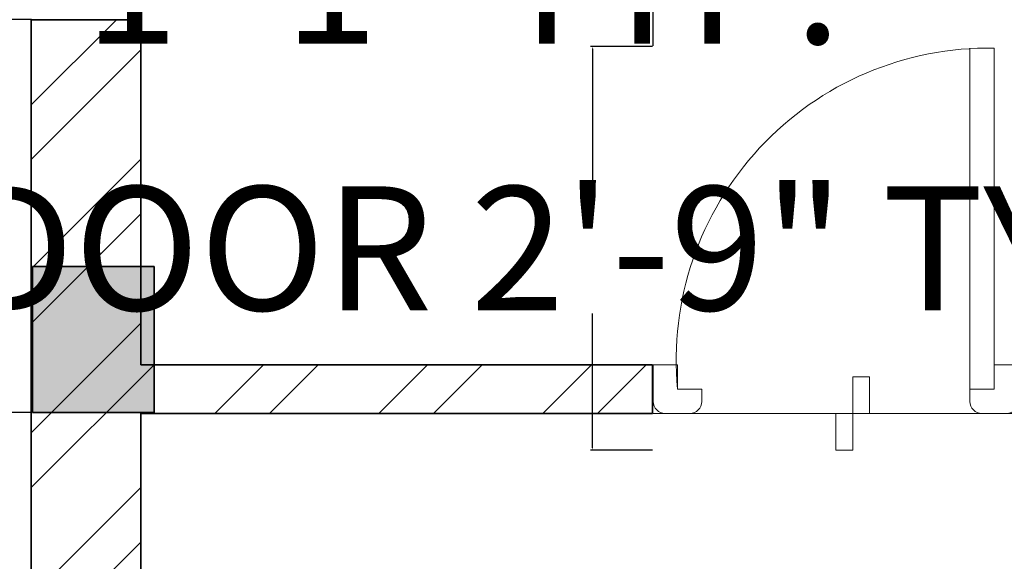
# Model space of a CAD drawing. Units: inches. Extents: x 1812 to 2791, y 2306 to 2959.
# Tile 6 of 8: x 2453 to 2534, y 2748 to 2793. Entities that reach past the tile are written whole.
import ezdxf

# ---------------------------------------------------------------- set-up
doc = ezdxf.new("R2010")
doc.units = ezdxf.units.IN
doc.layers.get('Defpoints').update_dxf_attribs({"lineweight": 50})
for name, color, linetype, lineweight in [('A-ANNO-DIMS', 2, 'Continuous', 18), ('A-COLS', 7, 'Continuous', 35), ('A-WALL-PATT', 8, 'Continuous', 13), ('A_FUR 1', 5, 'Continuous', 5), ('DOORS', 4, 'Continuous', 18), ('WALL', 7, 'Continuous', 35)]:
    doc.layers.add(name, color=color, linetype=linetype, lineweight=lineweight)
doc.styles.get("Standard").update_dxf_attribs({"font": 'arial.ttf'})
doc.dimstyles.get("Standard").update_dxf_attribs({"dimtxt": 10.18, "dimasz": 0.18, "dimexe": 0.18, "dimexo": 0.0625, "dimgap": 0.09, "dimtad": 0, "dimtih": 1, "dimtoh": 1, "dimdec": 0, "dimzin": 0, "dimdsep": 46, "dimlunit": 3, "dimtxsty": 'Standard', "dimcen": 0.09, "dimadec": 0, "dimazin": 0, "dimtfac": 1, "dimtdec": 0, "dimtofl": 0, "dimtmove": 0, "dimatfit": 3, "dimfxl": 1, "dimtolj": 1, "dimtzin": 0, "dimarcsym": 0})

# ---------------------------------------------------------------- blocks, each defined once
blk = doc.blocks.new('ESTSET')
at = {"layer": 'A_FUR 1'}
for p, q in [((-10.44359699611232, 4.096573562603225), (-10.44359699611232, 32.09657356260323)), ((-8.44359699611232, 4.096573562603225), (-8.44359699611232, 32.09657356260323)), ((-36.44359699611232, 6.096573562603225), (-36.44359699611232, 3.096573562603225)), ((-34.44359699611232, 6.096573562603225), (-36.44359699611232, 6.096573562603225)), ((-34.44359699611232, 4.096573562603225), (-34.44359699611232, 6.096573562603225)), ((-34.44359699611232, 4.096573562603225), (-34.44359699611232, 6.096573562603225)), ((-8.44359699611232, 4.096573562603225), (-8.44359699611232, 6.096573562603225)), ((-8.44359699611232, 6.096573562603225), (-6.443596996112319, 6.096573562603225)), ((-8.44359699611232, 4.096573562603225), (-8.44359699611232, 6.096573562603225)), ((-6.443596996112319, 6.096573562603225), (-6.443596996112319, 3.096573562603225)), ((-32.44359699611232, 4.096573562603225), (-34.44359699611232, 4.096573562603225)), ((-32.44359699611232, 4.096573562603225), (-34.44359699611232, 4.096573562603225)), ((-32.44359699611232, 3.096573562603225), (-32.44359699611232, 4.096573562603225)), ((-10.44359699611232, 3.096573562603225), (-10.44359699611232, 4.096573562603225)), ((-10.44359699611232, 4.096573562603225), (-8.44359699611232, 4.096573562603225)), ((-10.44359699611232, 4.096573562603225), (-8.44359699611232, 4.096573562603225)), ((-6.443596996112319, 2.096573562601521), (-36.4435969961196, 2.09657356260334)), ((-35.44359699611232, 2.096573562603225), (-33.44359699611232, 2.096573562603225)), ((-7.443596996112319, 2.096573562603225), (-9.44359699611232, 2.096573562603225))]:
    blk.add_line(p, q, dxfattribs=at)
for points in [[(-21.44359699614506, 2.09657356260334), (-18.67227073841423, 2.09657356260334), (-18.67227073841423, 5.101808480258228), (-20.05793386727964, 5.101808480258228)], [(-20.05793386727964, 5.101808480258228), (-20.05793386727964, -0.9086613550515485)], [(-21.44359699614506, 2.09657356260334), (-21.44359699614506, -0.9086613550515485), (-20.05793386727964, -0.9086613550515485)]]:
    blk.add_lwpolyline(points, dxfattribs=at)
for centre, radius, start, end in [((-8.908777800232201, 6.457098594999479), 25.64369454261379, 88.96058819788949, 185.2816045955121), ((-35.44359699611232, 3.096573562603225), 1, 180, 270), ((-33.44359699611232, 3.096573562603225), 1, 270, 0), ((-9.44359699611232, 3.096573562603225), 1, 180, 270), ((-7.443596996112319, 3.096573562603225), 1, 270, 0)]:
    blk.add_arc(centre, radius, start, end, dxfattribs=at)
blk = doc.blocks.new('COL')
at = {"transparency": 33554687}
h = blk.add_hatch(color=256, dxfattribs=at)
h.dxf.hatch_style = 1
h.paths.add_polyline_path([(2424.397880689844, 2829.240948453883), (2424.397880689844, 2839.240948453883), (2412.397880689843, 2839.240948453883), (2412.397880689843, 2829.240948453883)])
for p, q in [((2412.397880689843, 2839.240948453883), (2424.397880689844, 2839.240948453883)), ((2412.397880689843, 2839.240948453883), (2412.397880689843, 2829.240948453882)), ((2424.397880689844, 2839.240948453883), (2424.397880689844, 2829.240948453883)), ((2412.397880689843, 2829.240948453883), (2424.397880689844, 2829.240948453883))]:
    blk.add_line(p, q)
blk = doc.blocks.new('*D48')
at = {"layer": 'A-ANNO-DIMS', "color": 0, "lineweight": -2, "transparency": 16777216}
for p, q in [((2454.200753859796, 2816.957881357629), (2450.483253859797, 2816.957881357629)), ((2450.663253859797, 2816.777881357629), (2450.663253859797, 2810.245514372636)), ((2450.663253859797, 2793.137881357629), (2450.663253859797, 2799.670248342622)), ((2454.200753859796, 2792.957881357629), (2450.483253859797, 2792.957881357629))]:
    blk.add_line(p, q, dxfattribs=at)
at = {"layer": 'A-ANNO-DIMS', "color": 0, "transparency": 16777216}
for points in [[(2450.633253859797, 2816.777881357629), (2450.693253859797, 2816.777881357629), (2450.663253859797, 2816.957881357629)], [(2450.633253859797, 2793.137881357629), (2450.693253859797, 2793.137881357629), (2450.663253859797, 2792.957881357629)]]:
    blk.add_solid(points, dxfattribs=at)
at = {"layer": 'Defpoints', "color": 0, "transparency": 16777216}
for p in [(2450.663253859797, 2816.957881357629), (2454.263253859796, 2816.957881357629), (2454.263253859796, 2792.957881357629)]:
    blk.add_point(p, dxfattribs=at)
at = {"layer": 'A-ANNO-DIMS', "color": 0, "transparency": 16777216, "insert": (2450.663253859797, 2804.957881357628), "char_height": 10.18, "attachment_point": 5}
blk.add_mtext('\\A1;VENT 2\'-0" TYP.', dxfattribs=at)
blk = doc.blocks.new('*D58')
at = {"layer": 'A-ANNO-DIMS', "color": 0, "lineweight": -2, "transparency": 16777216}
for p, q in [((2533.666907414658, 2818.774380578327), (2536.746255119824, 2818.774380578327)), ((2536.566255119824, 2818.594380578328), (2536.566255119824, 2814.255156531551)), ((2536.566255119824, 2799.20872921056), (2536.566255119824, 2803.547953257336)), ((2533.666907414658, 2799.02872921056), (2536.746255119824, 2799.02872921056))]:
    blk.add_line(p, q, dxfattribs=at)
at = {"layer": 'A-ANNO-DIMS', "color": 0, "transparency": 16777216}
for points in [[(2536.536255119824, 2818.594380578328), (2536.596255119824, 2818.594380578328), (2536.566255119824, 2818.774380578327)], [(2536.536255119824, 2799.20872921056), (2536.596255119824, 2799.20872921056), (2536.566255119824, 2799.02872921056)]]:
    blk.add_solid(points, dxfattribs=at)
at = {"layer": 'Defpoints', "color": 0, "transparency": 16777216}
for p in [(2533.604407414657, 2818.774380578327), (2533.604407414657, 2799.02872921056), (2536.566255119824, 2799.02872921056)]:
    blk.add_point(p, dxfattribs=at)
at = {"layer": 'A-ANNO-DIMS', "color": 0, "transparency": 16777216, "insert": (2536.566255119824, 2808.901554894443), "char_height": 10.18, "attachment_point": 5}
blk.add_mtext('\\A1;BASIN 1\'-7 1/2" TYP.', dxfattribs=at)
blk = doc.blocks.new('*D59')
at = {"layer": 'A-ANNO-DIMS', "color": 0, "lineweight": -2, "transparency": 16777216}
for p, q in [((2520.440639836141, 2798.966229210559), (2520.440639836141, 2795.886881505393)), ((2533.604407414657, 2798.966229210559), (2533.604407414657, 2795.886881505393)), ((2520.440639836141, 2796.066881505393), (2520.260639836141, 2796.066881505393)), ((2533.424407414657, 2796.066881505393), (2520.620639836141, 2796.066881505393))]:
    blk.add_line(p, q, dxfattribs=at)
at = {"layer": 'A-ANNO-DIMS', "color": 0, "transparency": 16777216}
for points in [[(2520.620639836141, 2796.096881505393), (2520.620639836141, 2796.036881505393), (2520.440639836141, 2796.066881505393)], [(2533.424407414657, 2796.096881505393), (2533.424407414657, 2796.036881505393), (2533.604407414657, 2796.066881505393)]]:
    blk.add_solid(points, dxfattribs=at)
at = {"layer": 'Defpoints', "color": 0, "transparency": 16777216}
for p in [(2520.440639836141, 2799.028729210559), (2533.604407414657, 2799.028729210559), (2520.440639836141, 2796.066881505393)]:
    blk.add_point(p, dxfattribs=at)
at = {"layer": 'A-ANNO-DIMS', "color": 0, "transparency": 16777216, "insert": (2489.623695770657, 2796.066881505393), "char_height": 10.18, "attachment_point": 5}
blk.add_mtext('\\A1;1\'-1" TYP.', dxfattribs=at)
blk = doc.blocks.new('*D60')
at = {"layer": 'A-ANNO-DIMS', "color": 0, "lineweight": -2, "transparency": 16777216}
for p, q in [((2505.177694196558, 2790.74953182163), (2500.089565400664, 2790.74953182163)), ((2500.269565400663, 2790.56953182163), (2500.269565400663, 2779.537842838497)), ((2500.269565400663, 2757.792006515665), (2500.269565400663, 2768.823695498797)), ((2505.177694196558, 2757.612006515665), (2500.089565400664, 2757.612006515665))]:
    blk.add_line(p, q, dxfattribs=at)
at = {"layer": 'A-ANNO-DIMS', "color": 0, "transparency": 16777216}
for points in [[(2500.239565400664, 2790.56953182163), (2500.299565400664, 2790.56953182163), (2500.269565400663, 2790.74953182163)], [(2500.239565400664, 2757.792006515665), (2500.299565400664, 2757.792006515665), (2500.269565400663, 2757.612006515665)]]:
    blk.add_solid(points, dxfattribs=at)
at = {"layer": 'Defpoints', "color": 0, "transparency": 16777216}
for p in [(2500.269565400663, 2790.74953182163), (2505.240194196558, 2790.74953182163), (2505.240194196558, 2757.612006515665)]:
    blk.add_point(p, dxfattribs=at)
at = {"layer": 'A-ANNO-DIMS', "color": 0, "transparency": 16777216, "insert": (2500.269565400663, 2774.180769168646), "char_height": 10.18, "attachment_point": 5}
blk.add_mtext('\\A1;DOOR 2\'-9" TYP.', dxfattribs=at)
blk = doc.blocks.new('*D61')
at = {"layer": 'A-ANNO-DIMS', "color": 0, "lineweight": -2, "transparency": 16777216}
for p, q in [((2505.240194196556, 2790.812031821629), (2505.240194196556, 2795.900160617524)), ((2505.420194196557, 2795.720160617524), (2535.060194196564, 2795.720160617524)), ((2535.240194196564, 2790.812031821629), (2535.240194196564, 2795.900160617524)), ((2535.240194196564, 2795.720160617524), (2535.420194196563, 2795.720160617524))]:
    blk.add_line(p, q, dxfattribs=at)
at = {"layer": 'A-ANNO-DIMS', "color": 0, "transparency": 16777216}
for points in [[(2505.420194196557, 2795.750160617524), (2505.420194196557, 2795.690160617523), (2505.240194196556, 2795.720160617524)], [(2535.060194196564, 2795.750160617524), (2535.060194196564, 2795.690160617523), (2535.240194196564, 2795.720160617524)]]:
    blk.add_solid(points, dxfattribs=at)
at = {"layer": 'Defpoints', "color": 0, "transparency": 16777216}
for p in [(2535.240194196564, 2795.720160617524), (2505.240194196556, 2790.749531821629), (2535.240194196564, 2790.749531821629)]:
    blk.add_point(p, dxfattribs=at)
at = {"layer": 'A-ANNO-DIMS', "color": 0, "transparency": 16777216, "insert": (2566.623079599019, 2795.720160617524), "char_height": 10.18, "attachment_point": 5}
blk.add_mtext('\\A1;2\'-6" TYP.', dxfattribs=at)
blk = doc.blocks.new('*D64')
at = {"layer": 'A-ANNO-DIMS', "color": 0, "lineweight": -2, "transparency": 16777216}
for p, q in [((2499.736887761388, 2721.901978502181), (2499.736887761388, 2724.667753417118)), ((2499.916887761388, 2724.487753417118), (2517.212053860968, 2724.487753417118)), ((2517.392053860968, 2721.901978502181), (2517.392053860968, 2724.667753417118)), ((2517.392053860968, 2724.487753417118), (2517.572053860968, 2724.487753417118))]:
    blk.add_line(p, q, dxfattribs=at)
at = {"layer": 'A-ANNO-DIMS', "color": 0, "transparency": 16777216}
for points in [[(2499.916887761388, 2724.517753417118), (2499.916887761388, 2724.457753417118), (2499.736887761388, 2724.487753417118)], [(2517.212053860968, 2724.517753417118), (2517.212053860968, 2724.457753417118), (2517.392053860968, 2724.487753417118)]]:
    blk.add_solid(points, dxfattribs=at)
at = {"layer": 'Defpoints', "color": 0, "transparency": 16777216}
for p in [(2517.392053860968, 2724.487753417118), (2499.736887761388, 2721.839478502181), (2517.392053860968, 2721.839478502181)]:
    blk.add_point(p, dxfattribs=at)
at = {"layer": 'A-ANNO-DIMS', "color": 0, "transparency": 16777216, "insert": (2601.369291241595, 2724.487753417118), "char_height": 10.18, "attachment_point": 5}
blk.add_mtext('\\A1;END CHAIR 1\'-5 1/2" TYP.', dxfattribs=at)
blk = doc.blocks.new('*D73')
at = {"layer": 'A-ANNO-DIMS', "color": 0, "lineweight": -2, "transparency": 16777216}
for p, q in [((2454.218562000001, 2760.694666000001), (2428.586486000002, 2760.694666000001)), ((2428.766486000002, 2760.514666000001), (2428.766486000002, 2692.848797196454)), ((2428.766486000002, 2614.781264000001), (2428.766486000002, 2682.447132803548)), ((2454.176191000001, 2614.601264000001), (2428.586486000002, 2614.601264000001))]:
    blk.add_line(p, q, dxfattribs=at)
at = {"layer": 'A-ANNO-DIMS', "color": 0, "transparency": 16777216}
for points in [[(2428.736486000002, 2760.514666000001), (2428.796486000002, 2760.514666000001), (2428.766486000002, 2760.694666000001)], [(2428.736486000002, 2614.781264000001), (2428.796486000002, 2614.781264000001), (2428.766486000002, 2614.601264000001)]]:
    blk.add_solid(points, dxfattribs=at)
at = {"layer": 'Defpoints', "color": 0, "transparency": 16777216}
for p in [(2428.766486000002, 2760.694666000001), (2454.281062000001, 2760.694666000001), (2454.238691000001, 2614.601264000001)]:
    blk.add_point(p, dxfattribs=at)
at = {"layer": 'A-ANNO-DIMS', "color": 0, "transparency": 16777216, "insert": (2428.766486000002, 2687.647965), "char_height": 10.18, "attachment_point": 5}
blk.add_mtext('\\A1;12\'-2"', dxfattribs=at)

msp = doc.modelspace()

# ---------------------------------------------------------------- hatches: boundary and pattern name
at = {"layer": 'A-WALL-PATT'}
h = msp.add_hatch(dxfattribs=at)
h.set_pattern_fill('ANSI32', color=256)
h.set_pattern_definition([(45, (563.8057507655523, 20.01067828916757), (-6.735192090801865, 6.735192090801866), []), (45, (568.2958807655523, 20.01067828916757), (-6.735192090801865, 6.735192090801866), [])])
h.paths.add_polyline_path([(2694.192292649419, 2437.613622010101), (2683.499516441466, 2437.6136220101), (2683.499516441466, 2788.569354872347), (2685.192292649419, 2788.569354872347), (2685.192292649419, 2821.63505754476), (2685.125860943268, 2869.374403893766), (2685.125860943268, 2821.63505754476), (2694.192292649419, 2821.63505754476)])
h.paths.add_polyline_path([(2587.192292649419, 2446.613622010096), (2463.19229264942, 2446.613622010089), (2463.19229264942, 2473.613622010101), (2515.608214234135, 2473.613622010101), (2515.608214234135, 2477.6136220101), (2463.19229264942, 2477.6136220101), (2463.19229264942, 2610.6136220101), (2523.737487215154, 2610.613622010101), (2523.737487215154, 2614.613622010101), (2463.19229264942, 2614.6136220101), (2463.19229264942, 2654.536135698824), (2454.192292649419, 2654.536135698824), (2454.192292649419, 2437.613622010101), (2587.192292649419, 2437.613622010101)])
h.paths.add_polyline_path([(2683.499516441466, 2446.6136220101), (2676.19229264942, 2446.6136220101), (2676.192292649419, 2437.6136220101), (2683.499516441466, 2437.613622010101)])
h.paths.add_polyline_path([(2463.192292649419, 2760.6136220101), (2505.192292649419, 2760.6136220101), (2505.192292649419, 2764.6136220101), (2463.192292649419, 2764.6136220101), (2463.192292649419, 2792.952050683902), (2454.192292649419, 2792.952050683902), (2454.192292649419, 2702.536135698824), (2463.016486285651, 2702.536135698824), (2463.016486285651, 2702.649195550402)])
h.paths.add_polyline_path([(2539.192292649419, 2858.613622010101), (2463.192292649419, 2858.6136220101), (2463.192292649419, 2876.345134993912), (2454.192292649419, 2876.345134993912), (2454.19229264942, 2816.957881357627), (2463.192292649419, 2816.957881357627), (2463.192292649419, 2854.6136220101), (2535.192292649419, 2854.613622010101), (2535.192292649419, 2760.6136220101), (2539.192292649419, 2760.6136220101)])
h.paths.add_polyline_path([(2683.499516441466, 2917.613622010101), (2454.192292649419, 2917.613622010101), (2454.192292649419, 2900.372408669677), (2463.192292649419, 2900.372408669677), (2463.192292649419, 2908.6136220101), (2683.499516441466, 2908.613622010101)])
h.paths.add_polyline_path([(2694.192292649419, 2917.613622010101), (2683.499516441466, 2917.613622010101), (2683.499516441466, 2908.613622010101), (2685.192292649419, 2908.613622010101), (2685.192292649419, 2869.63505754476), (2694.192292649419, 2869.63505754476)])

# ---------------------------------------------------------------- linework, layer by layer
at = {"layer": 'WALL'}
for p, q in [((2454.192292649419, 2702.536135698824), (2454.192292649419, 2792.952050683902)), ((2463.192292649419, 2792.952050683902), (2454.192292649419, 2792.952050683902)), ((2463.192292649419, 2764.6136220101), (2463.192292649419, 2792.952050683902)), ((2463.19229264942, 2764.6136220101), (2505.192292649419, 2764.6136220101)), ((2505.192292649419, 2760.6136220101), (2505.192292649419, 2764.613622010101)), ((2463.19229264942, 2760.6136220101), (2505.192292649419, 2760.6136220101)), ((2463.19229264942, 2702.536135698824), (2463.192292649419, 2760.6136220101))]:
    msp.add_line(p, q, dxfattribs=at)

# ---------------------------------------------------------------- block references
at = {"layer": 'A-COLS', "rotation": 270}
msp.add_blockref('COL', (-374.9598863167703, 5185.092546519973), dxfattribs=at)
at = {"layer": 'DOORS'}
msp.add_blockref('ESTSET', (2541.683791192676, 2758.520667870716), dxfattribs=at)

# ---------------------------------------------------------------- dimensions: what is measured, and where the dimension line sits
at = {"layer": 'A-ANNO-DIMS'}
for base, p1, p2, angle, text, picture, middle in [((2536.566255119824, 2799.02872921056), (2533.604407414657, 2818.774380578327), (2533.604407414657, 2799.028729210559), 270, 'BASIN <> TYP.', '*D58', (2536.566255119824, 2808.901554894443)), ((2450.663253859797, 2816.957881357629), (2454.263253859795, 2792.957881357628), (2454.263253859795, 2816.957881357629), 90, 'VENT <> TYP.', '*D48', (2450.663253859797, 2804.957881357628)), ((2520.440639836141, 2796.066881505393), (2533.604407414657, 2799.028729210559), (2520.440639836141, 2799.028729210559), 180, '<> TYP.', '*D59', (2489.623695770657, 2796.066881505393)), ((2500.269565400663, 2790.74953182163), (2505.240194196556, 2757.612006515664), (2505.240194196556, 2790.749531821629), 90, 'DOOR <> TYP.', '*D60', (2500.269565400663, 2774.180769168646))]:
    dim = msp.add_linear_dim(base=base, p1=p1, p2=p2, angle=angle, text=text, dimstyle='Standard', override={"dimdec": 1, "dimlfac": 1, "dimrnd": 0, "dimzin": 1, "dimdsep": 46, "dimlunit": 4, "dimfrac": 2}, dxfattribs=at)
    dim.commit()
    dim.dimension.update_dxf_attribs({"geometry": picture, "text_midpoint": middle})
for base, p1, p2, text, picture, middle in [((2535.240194196564, 2795.720160617524), (2505.240194196556, 2790.749531821629), (2535.240194196564, 2790.749531821629), '<> TYP.', '*D61', (2566.623079599019, 2795.720160617524)), ((2517.392053860968, 2724.487753417118), (2499.736887761388, 2721.839478502181), (2517.392053860968, 2721.839478502181), 'END CHAIR <> TYP.', '*D64', (2601.369291241595, 2724.487753417118))]:
    dim = msp.add_linear_dim(base=base, p1=p1, p2=p2, text=text, dimstyle='Standard', override={"dimdec": 1, "dimlfac": 1, "dimrnd": 0, "dimzin": 1, "dimdsep": 46, "dimlunit": 4, "dimfrac": 2}, dxfattribs=at)
    dim.commit()
    dim.dimension.update_dxf_attribs({"geometry": picture, "text_midpoint": middle})
dim = msp.add_linear_dim(base=(2428.766486000002, 2760.694666000001), p1=(2454.238691, 2614.601264), p2=(2454.281062, 2760.694666), angle=90, dimstyle='Standard', override={"dimdec": 1, "dimlfac": 1, "dimrnd": 0, "dimzin": 1, "dimdsep": 46, "dimlunit": 4, "dimfrac": 2}, dxfattribs=at)
dim.commit()
dim.dimension.update_dxf_attribs({"geometry": '*D73', "text_midpoint": (2428.766486000002, 2687.647965)})

doc.saveas('drawing.dxf')
